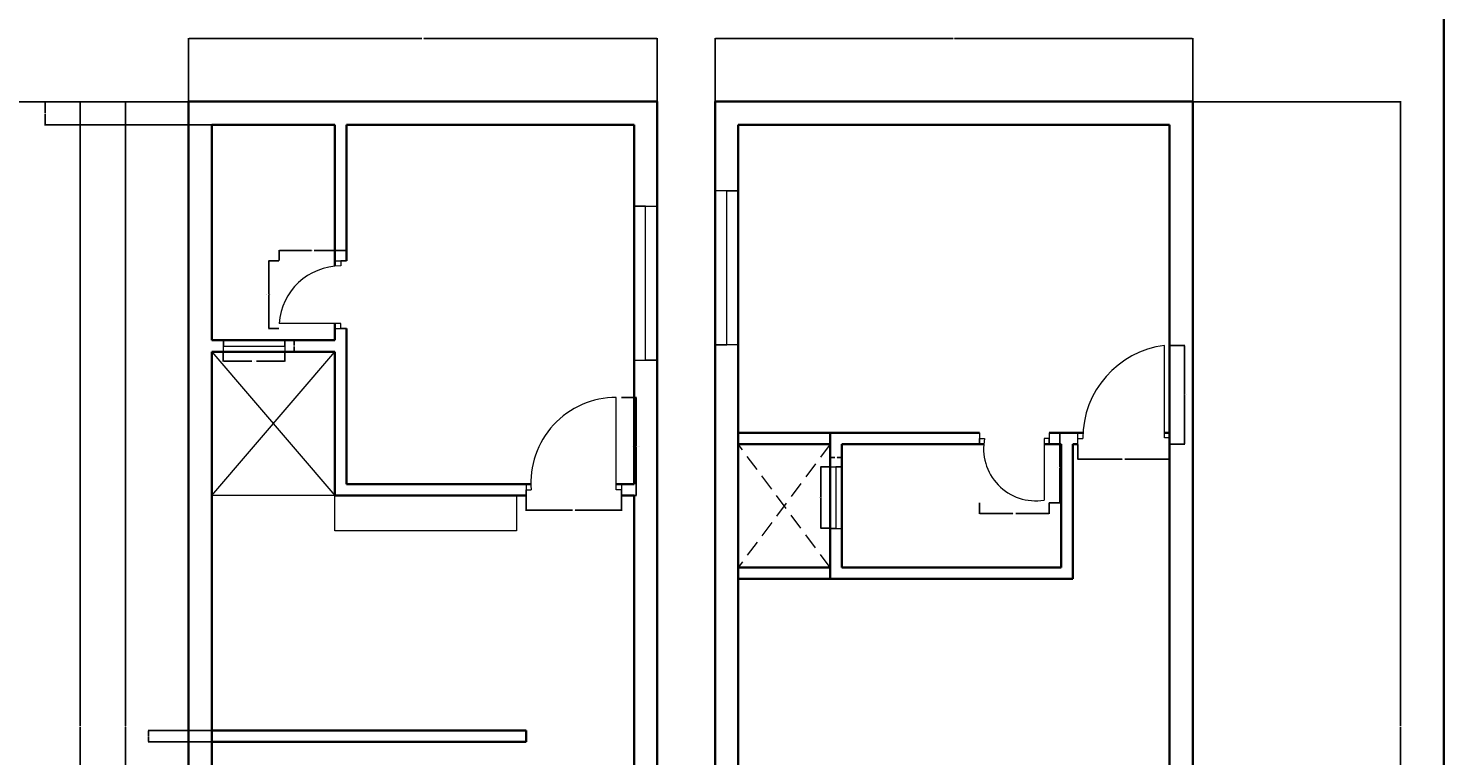
# Model space of a CAD drawing. Units: inches. Extents: x 2169 to 3181, y 1824 to 2912.
# Tile 4 of 5: x 2630 to 3181, y 2163 to 2446. Entities that reach past the tile are written whole.
import ezdxf

# ---------------------------------------------------------------- set-up
doc = ezdxf.new("R2010")
doc.units = ezdxf.units.IN
doc.linetypes.add('DASHED2', pattern=[9.525, 6.35, -3.175])
for name, color, linetype, lineweight in [('A-ANNO-DIMS', 2, 'Continuous', 18), ('A-ANNO-TTLB', 7, 'Continuous', 35), ('A-DOOR', 3, 'Continuous', 18), ('A-FLOR-CASE', 8, 'Continuous', 18), ('A-FLOR-OPEN', 7, 'Continuous', 18), ('A-FLOR-OPEN-OVHD', 253, 'DASHED2', 13), ('A-GLAZ', 4, 'Continuous', 18), ('A-WALL', 7, 'Continuous', 35)]:
    doc.layers.add(name, color=color, linetype=linetype, lineweight=lineweight)
doc.styles.get("Standard").update_dxf_attribs({"font": 'arial.ttf'})
doc.dimstyles.get("Standard").update_dxf_attribs({"dimtxt": 0.18, "dimasz": 0.18, "dimexe": 0.18, "dimexo": 0.0625, "dimgap": 0.09, "dimtad": 0, "dimtih": 1, "dimtoh": 1, "dimdec": 4, "dimzin": 0, "dimdsep": 46, "dimtxsty": 'Standard', "dimcen": 0.09, "dimadec": 0, "dimazin": 0, "dimtfac": 1, "dimtdec": 4, "dimtofl": 0, "dimtmove": 0, "dimatfit": 3, "dimfxl": 1, "dimtolj": 1, "dimtzin": 0, "dimarcsym": 0})

# ---------------------------------------------------------------- blocks, each defined once
blk = doc.blocks.new('DOOR-BED-G-36IN')
for p, q in [((0, 0), (0, 36)), ((-35.15, 2.25), (-35.15, -2.25)), ((2, 2.25), (2, -2.25)), ((-35.15, -2.25), (-35.15, 0)), ((-35.15, 0), (-33.15, 0)), ((2, 0), (0, 0)), ((2, -2.25), (2, 0))]:
    blk.add_line(p, q)
blk.add_arc((0, 2.74), 33.26, 90, 184.7229)
blk = doc.blocks.new('DOOR-BATH-G-24IN')
for p, q in [((-2.25, 24.37), (2.25, 24.37)), ((2.25, 24.37), (0, 24.37)), ((0, 24.37), (0, 22.37)), ((0, 0), (-24, 0)), ((0, -2), (0, 0)), ((-2.25, -2), (-2.25, -2)), ((-2.25, -2), (2.25, -2)), ((2.25, -2), (0, -2))]:
    blk.add_line(p, q)
blk.add_arc((0, -1.69), 24.06, 90, 175.9745)
blk = doc.blocks.new('DOOR-BATH-U-24IN')
for p, q in [((-25.15, 2.25), (-25.15, -2.25)), ((2, 2.25), (2, -2.25)), ((-25.15, -2.25), (-25.15, 0)), ((-25.15, 0), (-23.15, 0)), ((2, 0), (0, 0)), ((0, 0), (0, -24)), ((2, -2.25), (2, 0))]:
    blk.add_line(p, q)
blk.add_arc((-3.27, -3.99), 20.28, 168.6528, 279.2746)
blk = doc.blocks.new('DOOR-BED-U-36IN')
for p, q in [((0, 0), (0, 36)), ((-33.79, -2.49), (-33.79, 2.01)), ((-33.79, 2.01), (-33.79, 2.01)), ((2, 0), (0, 0)), ((-33.79, -0.24), (-31.79, -0.24)), ((-33.79, -2.49), (-33.79, -2.49))]:
    blk.add_line(p, q)
blk.add_arc((4.76, -0.24), 36.56, 97.4851, 180)
blk = doc.blocks.new('WIN-60IN')
for p, q in [((4.5, 60), (0, 60)), ((0, 60), (9, 60)), ((4.5, 0), (4.5, 60)), ((0, 0), (9, 0)), ((9, 0), (4.5, 0)), ((9, 0), (9, 0))]:
    blk.add_line(p, q)
blk = doc.blocks.new('VENT-24IN-G')
for p, q in [((0, 0), (0, 4.5)), ((0, 4.5), (0, 2.25)), ((0, 2.25), (24, 2.25)), ((24, 2.25), (24, 4.5)), ((24, 4.5), (24, 0))]:
    blk.add_line(p, q)
blk = doc.blocks.new('VENT-24IN-U')
for p, q in [((0, 24), (0, 24)), ((0, 24), (4.5, 24)), ((4.5, 24), (2.25, 24)), ((2.25, 24), (2.25, 0)), ((2.25, 0), (0, 0)), ((0, 0), (4.5, 0))]:
    blk.add_line(p, q)
blk = doc.blocks.new('*D23')
at = {"layer": 'A-ANNO-DIMS', "color": 0, "lineweight": -2, "transparency": 16777216}
for p, q in [((2705.49, 2319.83), (2705.49, 2316.11)), ((2705.67, 2316.29), (2716.59, 2316.29)), ((2729.31, 2316.29), (2718.4, 2316.29)), ((2729.49, 2319.83), (2729.49, 2316.11))]:
    blk.add_line(p, q, dxfattribs=at)
at = {"layer": 'A-ANNO-DIMS', "color": 0, "transparency": 16777216}
for points in [[(2705.67, 2316.32), (2705.67, 2316.26), (2705.49, 2316.29)], [(2729.31, 2316.32), (2729.31, 2316.26), (2729.49, 2316.29)]]:
    blk.add_solid(points, dxfattribs=at)
at = {"layer": 'Defpoints', "color": 0, "transparency": 16777216}
for p in [(2705.49, 2319.89), (2729.49, 2319.89), (2729.49, 2316.29)]:
    blk.add_point(p, dxfattribs=at)
at = {"layer": 'A-ANNO-DIMS', "color": 0, "transparency": 16777216, "insert": (2717.49, 2316.29), "char_height": 0.18, "attachment_point": 5}
blk.add_mtext('\\A1;VENT 24 TYP.', dxfattribs=at)
blk = doc.blocks.new('*D24')
at = {"layer": 'A-ANNO-DIMS', "color": 0, "lineweight": -2, "transparency": 16777216}
for p, q in [((2729.56, 2324.39), (2733.27, 2324.39)), ((2733.09, 2324.21), (2733.09, 2322.32)), ((2733.09, 2320.07), (2733.09, 2321.96)), ((2729.56, 2319.89), (2733.27, 2319.89))]:
    blk.add_line(p, q, dxfattribs=at)
at = {"layer": 'A-ANNO-DIMS', "color": 0, "transparency": 16777216}
for points in [[(2733.06, 2324.21), (2733.12, 2324.21), (2733.09, 2324.39)], [(2733.06, 2320.07), (2733.12, 2320.07), (2733.09, 2319.89)]]:
    blk.add_solid(points, dxfattribs=at)
at = {"layer": 'Defpoints', "color": 0, "transparency": 16777216}
for p in [(2729.49, 2324.39), (2733.09, 2324.39), (2729.49, 2319.89)]:
    blk.add_point(p, dxfattribs=at)
at = {"layer": 'A-ANNO-DIMS', "color": 0, "transparency": 16777216, "insert": (2733.09, 2322.14), "char_height": 0.18, "attachment_point": 5}
blk.add_mtext('\\A1;5 TYP.', dxfattribs=at)
blk = doc.blocks.new('*D25')
at = {"layer": 'A-ANNO-DIMS', "color": 0, "lineweight": -2, "transparency": 16777216}
for p, q in [((2941.79, 2275.13), (2938.07, 2275.13)), ((2938.25, 2274.95), (2938.25, 2263.31)), ((2938.25, 2251.31), (2938.25, 2262.95)), ((2941.79, 2251.13), (2938.07, 2251.13))]:
    blk.add_line(p, q, dxfattribs=at)
at = {"layer": 'A-ANNO-DIMS', "color": 0, "transparency": 16777216}
for points in [[(2938.22, 2274.95), (2938.28, 2274.95), (2938.25, 2275.13)], [(2938.22, 2251.31), (2938.28, 2251.31), (2938.25, 2251.13)]]:
    blk.add_solid(points, dxfattribs=at)
at = {"layer": 'Defpoints', "color": 0, "transparency": 16777216}
for p in [(2938.25, 2275.13), (2941.85, 2275.13), (2941.85, 2251.13)]:
    blk.add_point(p, dxfattribs=at)
at = {"layer": 'A-ANNO-DIMS', "color": 0, "transparency": 16777216, "insert": (2938.25, 2263.13), "char_height": 0.18, "attachment_point": 5}
blk.add_mtext('\\A1;VENT 24 TYP.', dxfattribs=at)
blk = doc.blocks.new('*D26')
at = {"layer": 'A-ANNO-DIMS', "color": 0, "lineweight": -2, "transparency": 16777216}
for p, q in [((2941.85, 2275.19), (2941.85, 2278.91)), ((2942.03, 2278.73), (2943.64, 2278.73)), ((2946.17, 2278.73), (2944.56, 2278.73)), ((2946.35, 2275.19), (2946.35, 2278.91))]:
    blk.add_line(p, q, dxfattribs=at)
at = {"layer": 'A-ANNO-DIMS', "color": 0, "transparency": 16777216}
for points in [[(2942.03, 2278.76), (2942.03, 2278.7), (2941.85, 2278.73)], [(2946.17, 2278.76), (2946.17, 2278.7), (2946.35, 2278.73)]]:
    blk.add_solid(points, dxfattribs=at)
at = {"layer": 'Defpoints', "color": 0, "transparency": 16777216}
for p in [(2946.35, 2278.73), (2941.85, 2275.13), (2946.35, 2275.13)]:
    blk.add_point(p, dxfattribs=at)
at = {"layer": 'A-ANNO-DIMS', "color": 0, "transparency": 16777216, "insert": (2944.1, 2278.73), "char_height": 0.18, "attachment_point": 5}
blk.add_mtext('\\A1;5 TYP.', dxfattribs=at)
blk = doc.blocks.new('*D31')
at = {"layer": 'A-ANNO-DIMS', "color": 0, "lineweight": -2, "transparency": 16777216}
for p, q in [((2860.62, 2302.14), (2866.47, 2302.14)), ((2866.29, 2301.96), (2866.29, 2283.2)), ((2866.29, 2264.07), (2866.29, 2282.83)), ((2860.62, 2263.89), (2866.47, 2263.89))]:
    blk.add_line(p, q, dxfattribs=at)
at = {"layer": 'A-ANNO-DIMS', "color": 0, "transparency": 16777216}
for points in [[(2866.26, 2301.96), (2866.32, 2301.96), (2866.29, 2302.14)], [(2866.26, 2264.07), (2866.32, 2264.07), (2866.29, 2263.89)]]:
    blk.add_solid(points, dxfattribs=at)
at = {"layer": 'Defpoints', "color": 0, "transparency": 16777216}
for p in [(2860.56, 2302.14), (2866.29, 2302.14), (2860.56, 2263.89)]:
    blk.add_point(p, dxfattribs=at)
at = {"layer": 'A-ANNO-DIMS', "color": 0, "transparency": 16777216, "insert": (2866.29, 2283.02), "char_height": 0.18, "attachment_point": 5}
blk.add_mtext('\\A1;BEDROOM DOOR 38 TYP.', dxfattribs=at)
blk = doc.blocks.new('*D32')
at = {"layer": 'A-ANNO-DIMS', "color": 0, "lineweight": -2, "transparency": 16777216}
for p, q in [((2823.41, 2263.83), (2823.41, 2257.97)), ((2860.56, 2263.83), (2860.56, 2257.97)), ((2823.59, 2258.15), (2841.45, 2258.15)), ((2860.38, 2258.15), (2842.51, 2258.15))]:
    blk.add_line(p, q, dxfattribs=at)
at = {"layer": 'A-ANNO-DIMS', "color": 0, "transparency": 16777216}
for points in [[(2823.59, 2258.18), (2823.59, 2258.12), (2823.41, 2258.15)], [(2860.38, 2258.18), (2860.38, 2258.12), (2860.56, 2258.15)]]:
    blk.add_solid(points, dxfattribs=at)
at = {"layer": 'Defpoints', "color": 0, "transparency": 16777216}
for p in [(2823.41, 2263.89), (2860.56, 2263.89), (2860.56, 2258.15)]:
    blk.add_point(p, dxfattribs=at)
at = {"layer": 'A-ANNO-DIMS', "color": 0, "transparency": 16777216, "insert": (2841.98, 2258.15), "char_height": 0.18, "attachment_point": 5}
blk.add_mtext('\\A1;37 TYP.', dxfattribs=at)
blk = doc.blocks.new('*D33')
at = {"layer": 'A-ANNO-DIMS', "color": 0, "lineweight": -2, "transparency": 16777216}
for p, q in [((2727.14, 2355.37), (2723.07, 2355.37)), ((2723.25, 2355.19), (2723.25, 2342.37)), ((2723.25, 2329.18), (2723.25, 2342)), ((2727.14, 2329), (2723.07, 2329))]:
    blk.add_line(p, q, dxfattribs=at)
at = {"layer": 'A-ANNO-DIMS', "color": 0, "transparency": 16777216}
for points in [[(2723.22, 2355.19), (2723.28, 2355.19), (2723.25, 2355.37)], [(2723.22, 2329.18), (2723.28, 2329.18), (2723.25, 2329)]]:
    blk.add_solid(points, dxfattribs=at)
at = {"layer": 'Defpoints', "color": 0, "transparency": 16777216}
for p in [(2723.25, 2355.37), (2727.21, 2355.37), (2727.21, 2329)]:
    blk.add_point(p, dxfattribs=at)
at = {"layer": 'A-ANNO-DIMS', "color": 0, "transparency": 16777216, "insert": (2723.25, 2342.19), "char_height": 0.18, "attachment_point": 5}
blk.add_mtext('\\A1;WC DOOR 26 TYP.', dxfattribs=at)
blk = doc.blocks.new('*D34')
at = {"layer": 'A-ANNO-DIMS', "color": 0, "lineweight": -2, "transparency": 16777216}
for p, q in [((2727.21, 2355.44), (2727.21, 2359.51)), ((2727.39, 2359.33), (2739.8, 2359.33)), ((2753.28, 2359.33), (2740.86, 2359.33)), ((2753.46, 2355.44), (2753.46, 2359.51))]:
    blk.add_line(p, q, dxfattribs=at)
at = {"layer": 'A-ANNO-DIMS', "color": 0, "transparency": 16777216}
for points in [[(2727.39, 2359.36), (2727.39, 2359.3), (2727.21, 2359.33)], [(2753.28, 2359.36), (2753.28, 2359.3), (2753.46, 2359.33)]]:
    blk.add_solid(points, dxfattribs=at)
at = {"layer": 'Defpoints', "color": 0, "transparency": 16777216}
for p in [(2727.21, 2355.37), (2753.46, 2359.33), (2753.46, 2355.37)]:
    blk.add_point(p, dxfattribs=at)
at = {"layer": 'A-ANNO-DIMS', "color": 0, "transparency": 16777216, "insert": (2740.33, 2359.33), "char_height": 0.18, "attachment_point": 5}
blk.add_mtext('\\A1;26 TYP.', dxfattribs=at)
blk = doc.blocks.new('*D37')
at = {"layer": 'A-ANNO-DIMS', "color": 0, "lineweight": -2, "transparency": 16777216}
for p, q in [((3074.12, 2322.39), (3080.01, 2322.39)), ((3079.83, 2322.21), (3079.83, 2303.32)), ((3079.83, 2284.07), (3079.83, 2302.96)), ((3074.12, 2283.89), (3080.01, 2283.89))]:
    blk.add_line(p, q, dxfattribs=at)
at = {"layer": 'A-ANNO-DIMS', "color": 0, "transparency": 16777216}
for points in [[(3079.8, 2322.21), (3079.86, 2322.21), (3079.83, 2322.39)], [(3079.8, 2284.07), (3079.86, 2284.07), (3079.83, 2283.89)]]:
    blk.add_solid(points, dxfattribs=at)
at = {"layer": 'Defpoints', "color": 0, "transparency": 16777216}
for p in [(3074.05, 2322.39), (3079.83, 2322.39), (3074.05, 2283.89)]:
    blk.add_point(p, dxfattribs=at)
at = {"layer": 'A-ANNO-DIMS', "color": 0, "transparency": 16777216, "insert": (3079.83, 2303.14), "char_height": 0.18, "attachment_point": 5}
blk.add_mtext('\\A1;BEDROOM DOOR 38 TYP.', dxfattribs=at)
blk = doc.blocks.new('*D38')
at = {"layer": 'A-ANNO-DIMS', "color": 0, "lineweight": -2, "transparency": 16777216}
for p, q in [((3038.26, 2283.83), (3038.26, 2277.94)), ((3074.05, 2283.83), (3074.05, 2277.94)), ((3038.44, 2278.12), (3055.63, 2278.12)), ((3073.87, 2278.12), (3056.68, 2278.12))]:
    blk.add_line(p, q, dxfattribs=at)
at = {"layer": 'A-ANNO-DIMS', "color": 0, "transparency": 16777216}
for points in [[(3038.44, 2278.15), (3038.44, 2278.09), (3038.26, 2278.12)], [(3073.87, 2278.15), (3073.87, 2278.09), (3074.05, 2278.12)]]:
    blk.add_solid(points, dxfattribs=at)
at = {"layer": 'Defpoints', "color": 0, "transparency": 16777216}
for p in [(3038.26, 2283.89), (3074.05, 2283.89), (3074.05, 2278.12)]:
    blk.add_point(p, dxfattribs=at)
at = {"layer": 'A-ANNO-DIMS', "color": 0, "transparency": 16777216, "insert": (3056.16, 2278.12), "char_height": 0.18, "attachment_point": 5}
blk.add_mtext('\\A1;36 TYP.', dxfattribs=at)
blk = doc.blocks.new('*D39')
at = {"layer": 'A-ANNO-DIMS', "color": 0, "lineweight": -2, "transparency": 16777216}
for p, q in [((3027.22, 2288.39), (3031.44, 2288.39)), ((3031.26, 2288.21), (3031.26, 2274.91)), ((3031.26, 2261.25), (3031.26, 2274.55)), ((3027.22, 2261.07), (3031.44, 2261.07))]:
    blk.add_line(p, q, dxfattribs=at)
at = {"layer": 'A-ANNO-DIMS', "color": 0, "transparency": 16777216}
for points in [[(3031.23, 2288.21), (3031.29, 2288.21), (3031.26, 2288.39)], [(3031.23, 2261.25), (3031.29, 2261.25), (3031.26, 2261.07)]]:
    blk.add_solid(points, dxfattribs=at)
at = {"layer": 'Defpoints', "color": 0, "transparency": 16777216}
for p in [(3027.16, 2288.39), (3031.26, 2288.39), (3027.16, 2261.07)]:
    blk.add_point(p, dxfattribs=at)
at = {"layer": 'A-ANNO-DIMS', "color": 0, "transparency": 16777216, "insert": (3031.26, 2274.73), "char_height": 0.18, "attachment_point": 5}
blk.add_mtext('\\A1;WC DOOR 27 TYP.', dxfattribs=at)
blk = doc.blocks.new('*D40')
at = {"layer": 'A-ANNO-DIMS', "color": 0, "lineweight": -2, "transparency": 16777216}
for p, q in [((3000.01, 2261.01), (3000.01, 2256.79)), ((3027.16, 2261.01), (3027.16, 2256.79)), ((3000.19, 2256.97), (3013.06, 2256.97)), ((3026.98, 2256.97), (3014.12, 2256.97))]:
    blk.add_line(p, q, dxfattribs=at)
at = {"layer": 'A-ANNO-DIMS', "color": 0, "transparency": 16777216}
for points in [[(3000.19, 2257), (3000.19, 2256.94), (3000.01, 2256.97)], [(3026.98, 2257), (3026.98, 2256.94), (3027.16, 2256.97)]]:
    blk.add_solid(points, dxfattribs=at)
at = {"layer": 'Defpoints', "color": 0, "transparency": 16777216}
for p in [(3000.01, 2261.07), (3027.16, 2261.07), (3027.16, 2256.97)]:
    blk.add_point(p, dxfattribs=at)
at = {"layer": 'A-ANNO-DIMS', "color": 0, "transparency": 16777216, "insert": (3013.59, 2256.97), "char_height": 0.18, "attachment_point": 5}
blk.add_mtext('\\A1;27 TYP.', dxfattribs=at)
blk = doc.blocks.new('*D56')
at = {"layer": 'A-ANNO-DIMS', "color": 0, "lineweight": -2, "transparency": 16777216}
for p, q in [((2623.43, 2417.39), (2649.9, 2417.39)), ((2649.72, 2417.21), (2649.72, 2174.07)), ((2649.72, 1930.57), (2649.72, 2173.71)), ((2623.43, 1930.39), (2649.9, 1930.39))]:
    blk.add_line(p, q, dxfattribs=at)
at = {"layer": 'A-ANNO-DIMS', "color": 0, "transparency": 16777216}
for points in [[(2649.69, 2417.21), (2649.75, 2417.21), (2649.72, 2417.39)], [(2649.69, 1930.57), (2649.75, 1930.57), (2649.72, 1930.39)]]:
    blk.add_solid(points, dxfattribs=at)
at = {"layer": 'Defpoints', "color": 0, "transparency": 16777216}
for p in [(2623.37, 2417.39), (2649.72, 2417.39), (2623.37, 1930.39)]:
    blk.add_point(p, dxfattribs=at)
at = {"layer": 'A-ANNO-DIMS', "color": 0, "transparency": 16777216, "insert": (2649.72, 2173.89), "char_height": 0.18, "attachment_point": 5}
blk.add_mtext('\\A1;487', dxfattribs=at)
blk = doc.blocks.new('*D64')
at = {"layer": 'A-ANNO-DIMS', "color": 0, "lineweight": -2, "transparency": 16777216}
for p, q in [((2691.96, 2417.45), (2691.96, 2442.17)), ((2692.14, 2441.99), (2782.82, 2441.99)), ((2874.28, 2441.99), (2783.59, 2441.99)), ((2874.46, 2417.45), (2874.46, 2442.17))]:
    blk.add_line(p, q, dxfattribs=at)
at = {"layer": 'A-ANNO-DIMS', "color": 0, "transparency": 16777216}
for points in [[(2692.14, 2442.02), (2692.14, 2441.96), (2691.96, 2441.99)], [(2874.28, 2442.02), (2874.28, 2441.96), (2874.46, 2441.99)]]:
    blk.add_solid(points, dxfattribs=at)
at = {"layer": 'Defpoints', "color": 0, "transparency": 16777216}
for p in [(2874.46, 2441.99), (2691.96, 2417.39), (2874.46, 2417.39)]:
    blk.add_point(p, dxfattribs=at)
at = {"layer": 'A-ANNO-DIMS', "color": 0, "transparency": 16777216, "insert": (2783.21, 2441.99), "char_height": 0.18, "attachment_point": 5}
blk.add_mtext('\\A1;182.5', dxfattribs=at)
blk = doc.blocks.new('*D65')
at = {"layer": 'A-ANNO-DIMS', "color": 0, "lineweight": -2, "transparency": 16777216}
for p, q in [((2691.89, 2417.39), (2667.18, 2417.39)), ((2667.36, 2417.21), (2667.36, 2174.07)), ((2667.36, 1930.57), (2667.36, 2173.71)), ((2691.89, 1930.39), (2667.18, 1930.39))]:
    blk.add_line(p, q, dxfattribs=at)
at = {"layer": 'A-ANNO-DIMS', "color": 0, "transparency": 16777216}
for points in [[(2667.33, 2417.21), (2667.39, 2417.21), (2667.36, 2417.39)], [(2667.33, 1930.57), (2667.39, 1930.57), (2667.36, 1930.39)]]:
    blk.add_solid(points, dxfattribs=at)
at = {"layer": 'Defpoints', "color": 0, "transparency": 16777216}
for p in [(2667.36, 2417.39), (2691.96, 2417.39), (2691.96, 1930.39)]:
    blk.add_point(p, dxfattribs=at)
at = {"layer": 'A-ANNO-DIMS', "color": 0, "transparency": 16777216, "insert": (2667.36, 2173.89), "char_height": 0.18, "attachment_point": 5}
blk.add_mtext('\\A1;487', dxfattribs=at)
blk = doc.blocks.new('*D66')
at = {"layer": 'A-ANNO-DIMS', "color": 0, "lineweight": -2, "transparency": 16777216}
for p, q in [((2897.05, 2417.45), (2897.05, 2442.17)), ((2897.23, 2441.99), (2989.77, 2441.99)), ((3082.87, 2441.99), (2990.33, 2441.99)), ((3083.05, 2417.45), (3083.05, 2442.17))]:
    blk.add_line(p, q, dxfattribs=at)
at = {"layer": 'A-ANNO-DIMS', "color": 0, "transparency": 16777216}
for points in [[(2897.23, 2442.02), (2897.23, 2441.96), (2897.05, 2441.99)], [(3082.87, 2442.02), (3082.87, 2441.96), (3083.05, 2441.99)]]:
    blk.add_solid(points, dxfattribs=at)
at = {"layer": 'Defpoints', "color": 0, "transparency": 16777216}
for p in [(3083.05, 2441.99), (2897.05, 2417.39), (3083.05, 2417.39)]:
    blk.add_point(p, dxfattribs=at)
at = {"layer": 'A-ANNO-DIMS', "color": 0, "transparency": 16777216, "insert": (2990.05, 2441.99), "char_height": 0.18, "attachment_point": 5}
blk.add_mtext('\\A1;186', dxfattribs=at)
blk = doc.blocks.new('*D67')
at = {"layer": 'A-ANNO-DIMS', "color": 0, "lineweight": -2, "transparency": 16777216}
for p, q in [((3083.12, 2417.39), (3164.24, 2417.39)), ((3164.06, 2417.21), (3164.06, 2174.07)), ((3164.06, 1930.57), (3164.06, 2173.71)), ((3083.12, 1930.39), (3164.24, 1930.39))]:
    blk.add_line(p, q, dxfattribs=at)
at = {"layer": 'A-ANNO-DIMS', "color": 0, "transparency": 16777216}
for points in [[(3164.03, 2417.21), (3164.09, 2417.21), (3164.06, 2417.39)], [(3164.03, 1930.57), (3164.09, 1930.57), (3164.06, 1930.39)]]:
    blk.add_solid(points, dxfattribs=at)
at = {"layer": 'Defpoints', "color": 0, "transparency": 16777216}
for p in [(3083.05, 2417.39), (3164.06, 2417.39), (3083.05, 1930.39)]:
    blk.add_point(p, dxfattribs=at)
at = {"layer": 'A-ANNO-DIMS', "color": 0, "transparency": 16777216, "insert": (3164.06, 2173.89), "char_height": 0.18, "attachment_point": 5}
blk.add_mtext('\\A1;487', dxfattribs=at)
blk = doc.blocks.new('*D69')
at = {"layer": 'A-ANNO-DIMS', "color": 0, "lineweight": -2, "transparency": 16777216}
for p, q in [((2691.89, 2417.39), (2635.88, 2417.39)), ((2636.06, 2417.21), (2636.06, 2413.07)), ((2636.06, 2408.57), (2636.06, 2412.71)), ((2700.89, 2408.39), (2635.88, 2408.39))]:
    blk.add_line(p, q, dxfattribs=at)
at = {"layer": 'A-ANNO-DIMS', "color": 0, "transparency": 16777216}
for points in [[(2636.03, 2417.21), (2636.09, 2417.21), (2636.06, 2417.39)], [(2636.03, 2408.57), (2636.09, 2408.57), (2636.06, 2408.39)]]:
    blk.add_solid(points, dxfattribs=at)
at = {"layer": 'Defpoints', "color": 0, "transparency": 16777216}
for p in [(2691.96, 2417.39), (2636.06, 2408.39), (2700.96, 2408.39)]:
    blk.add_point(p, dxfattribs=at)
at = {"layer": 'A-ANNO-DIMS', "color": 0, "transparency": 16777216, "insert": (2636.06, 2412.89), "char_height": 0.18, "attachment_point": 5}
blk.add_mtext('\\A1;9', dxfattribs=at)
blk = doc.blocks.new('*D70')
at = {"layer": 'A-ANNO-DIMS', "color": 0, "lineweight": -2, "transparency": 16777216}
for p, q in [((2700.89, 2172.39), (2676.18, 2172.39)), ((2676.36, 2172.21), (2676.36, 2170.32)), ((2700.89, 2167.89), (2676.18, 2167.89)), ((2676.36, 2168.07), (2676.36, 2169.96))]:
    blk.add_line(p, q, dxfattribs=at)
at = {"layer": 'A-ANNO-DIMS', "color": 0, "transparency": 16777216}
for points in [[(2676.33, 2172.21), (2676.39, 2172.21), (2676.36, 2172.39)], [(2676.33, 2168.07), (2676.39, 2168.07), (2676.36, 2167.89)]]:
    blk.add_solid(points, dxfattribs=at)
at = {"layer": 'Defpoints', "color": 0, "transparency": 16777216}
for p in [(2676.36, 2172.39), (2700.96, 2172.39), (2700.96, 2167.89)]:
    blk.add_point(p, dxfattribs=at)
at = {"layer": 'A-ANNO-DIMS', "color": 0, "transparency": 16777216, "insert": (2676.36, 2170.14), "char_height": 0.18, "attachment_point": 5}
blk.add_mtext('\\A1;4.5', dxfattribs=at)

msp = doc.modelspace()

# ---------------------------------------------------------------- linework, layer by layer
at = {"layer": 'A-ANNO-TTLB'}
msp.add_lwpolyline([(2168.7598, 2912.462), (3180.8253, 2912.462), (3180.8253, 1823.5481), (2168.7598, 1823.5481)], close=True, dxfattribs=at)
at = {"layer": 'A-FLOR-CASE'}
msp.add_lwpolyline([(2748.9572, 2263.8924), (2819.6652, 2263.8924), (2819.6652, 2250.1381), (2748.9572, 2250.1381)], close=True, dxfattribs=at)
at = {"layer": 'A-FLOR-OPEN'}
for p, q in [((2700.9572, 2263.8924), (2748.9572, 2319.8924)), ((2700.9572, 2319.8924), (2748.9572, 2263.8924)), ((2748.9572, 2263.8924), (2700.9572, 2263.8924))]:
    msp.add_line(p, q, dxfattribs=at)
at = {"layer": 'A-FLOR-OPEN-OVHD'}
for p, q in [((2941.8523, 2283.8924), (2906.0534, 2235.8924)), ((2941.8523, 2235.8924), (2906.0534, 2283.8924)), ((2941.8523, 2273.085), (2941.8523, 2273.085))]:
    msp.add_line(p, q, dxfattribs=at)
at = {"layer": 'A-WALL'}
for p, q in [((2691.9572, 2417.3924), (2874.4572, 2417.3924)), ((2691.9572, 2417.3924), (2874.4572, 2417.3924)), ((2691.9572, 2417.3924), (2691.9572, 1930.3924)), ((2874.4572, 2417.3924), (2874.4572, 1930.3924)), ((2897.0534, 2417.3924), (3083.0534, 2417.3924)), ((2897.0534, 2417.3924), (2897.0534, 1930.3924)), ((3074.0534, 2417.3924), (3083.0534, 2417.3924)), ((3083.0534, 2417.3924), (3083.0534, 1930.3924)), ((2700.9572, 2408.3924), (2748.9572, 2408.3924)), ((2700.9572, 2408.3924), (2700.9572, 2324.3924)), ((2748.9572, 2408.3924), (2748.9572, 2353.2673)), ((2753.4572, 2408.3924), (2865.4572, 2408.3924)), ((2753.4572, 2408.3924), (2753.4572, 2355.3727)), ((2865.4572, 2408.3924), (2865.4572, 2268.3924)), ((2906.0534, 2408.3924), (3074.0534, 2408.3924)), ((2906.0534, 2408.3924), (2906.0534, 2023.8924)), ((2906.0534, 2408.3924), (3070.0534, 2408.3924)), ((2906.0534, 2408.3924), (3074.0534, 2408.3924)), ((3074.0534, 2408.3924), (3074.0534, 1930.3924)), ((2748.9572, 2331.0023), (2748.9572, 2324.3924)), ((2753.4572, 2329.0023), (2753.4572, 2268.3924)), ((2700.9572, 2324.3924), (2748.9572, 2324.3924)), ((2700.9572, 2319.8924), (2748.9572, 2319.8924)), ((2700.9572, 2319.8924), (2700.9572, 2023.8924)), ((2748.9572, 2319.8924), (2748.9572, 2263.8924)), ((2941.8523, 2288.3924), (2906.0534, 2288.3924)), ((2906.0534, 2288.3924), (2906.0534, 2283.8924)), ((2941.8523, 2288.3924), (3000.0137, 2288.3924)), ((2941.8523, 2288.3924), (2941.8523, 2231.3924)), ((2941.8523, 2288.3924), (3000.0137, 2288.3924)), ((3027.1608, 2288.3924), (3040.3285, 2288.3924)), ((3027.1608, 2288.3924), (3031.8523, 2288.3924)), ((3072.0534, 2288.3924), (3074.0534, 2288.3924)), ((2906.0534, 2283.8924), (2941.8523, 2283.8924)), ((2906.0534, 2283.8924), (2910.5534, 2283.8924)), ((2941.8523, 2283.8924), (2941.8523, 2231.3924)), ((2946.3523, 2283.8924), (3001.6921, 2283.8924)), ((2946.3523, 2283.8924), (2946.3523, 2235.8924)), ((3025.1608, 2283.8924), (3031.8523, 2283.8924)), ((3031.8523, 2283.8924), (3031.8523, 2235.8924)), ((3036.3523, 2283.8924), (3038.2592, 2283.8924)), ((3036.3523, 2231.3924), (3036.3523, 2283.8924)), ((2753.4572, 2268.3924), (2825.2991, 2268.3924)), ((2858.5569, 2268.3924), (2865.4572, 2268.3924)), ((2748.9572, 2263.8924), (2823.4085, 2263.8924)), ((2860.5569, 2263.8924), (2865.4572, 2263.8924)), ((2865.4572, 2263.8924), (2865.4572, 1930.3924)), ((2906.0534, 2231.3924), (2906.0534, 2235.8924)), ((2906.0534, 2235.8924), (2941.8523, 2235.8924)), ((2941.8523, 2235.8924), (2941.8523, 2235.8924)), ((2946.3523, 2235.8924), (3031.8523, 2235.8924)), ((2941.8523, 2231.3924), (2906.0534, 2231.3924)), ((2941.8523, 2231.3924), (3036.3523, 2231.3924)), ((3031.8523, 2231.3924), (3036.3523, 2231.3924)), ((2700.9572, 2172.3924), (2823.4085, 2172.3924)), ((2823.4085, 2172.3924), (2823.4085, 2167.8924)), ((2700.9572, 2167.8924), (2823.4085, 2167.8924))]:
    msp.add_line(p, q, dxfattribs=at)

# ---------------------------------------------------------------- block references
at = {"layer": 'A-DOOR'}
for name, p in [('DOOR-BATH-G-24IN', (2751.2072, 2331.0023)), ('DOOR-BED-U-36IN', (3072.0534, 2286.3872)), ('DOOR-BED-G-36IN', (2858.5569, 2266.1424)), ('DOOR-BATH-U-24IN', (3025.1608, 2286.1424))]:
    msp.add_blockref(name, p, dxfattribs=at)
at = {"layer": 'A-GLAZ', "extrusion": (0, 0, -1), "zscale": -1}
msp.add_blockref('WIN-60IN', (-2906.053, 2322.6361), dxfattribs=at)
at = {"layer": 'A-GLAZ'}
for name, p in [('WIN-60IN', (2865.4576, 2316.692)), ('VENT-24IN-G', (2705.4926, 2319.892)), ('VENT-24IN-U', (2941.8526, 2251.127))]:
    msp.add_blockref(name, p, dxfattribs=at)

# ---------------------------------------------------------------- dimensions: what is measured, and where the dimension line sits
at = {"layer": 'A-ANNO-DIMS'}
for base, p1, p2, override, picture, middle in [((2874.4572, 2441.9924), (2691.9572, 2417.3924), (2874.4572, 2417.3924), {"dimdec": 1, "dimlfac": 1, "dimrnd": 0, "dimzin": 0, "dimdsep": 46, "dimlunit": 2}, '*D64', (2783.2072, 2441.9924)), ((3083.0534, 2441.9924), (2897.0534, 2417.3924), (3083.0534, 2417.3924), {"dimdec": 0, "dimlfac": 1, "dimrnd": 0, "dimzin": 0, "dimdsep": 46, "dimlunit": 2}, '*D66', (2990.0534, 2441.9924))]:
    dim = msp.add_linear_dim(base=base, p1=p1, p2=p2, dimstyle='Standard', override=override, dxfattribs=at)
    dim.commit()
    dim.dimension.update_dxf_attribs({"geometry": picture, "text_midpoint": middle})
for base, p1, p2, override, picture, middle in [((2649.7198, 2417.3924), (2623.3698, 1930.3924), (2623.3698, 2417.3924), {"dimdec": 0, "dimlfac": 1, "dimrnd": 0, "dimzin": 0, "dimdsep": 46, "dimlunit": 2}, '*D56', (2649.7198, 2173.8924)), ((2636.0608, 2408.3924), (2691.9572, 2417.3924), (2700.9572, 2408.3924), {"dimdec": 0, "dimlfac": 1, "dimrnd": 0, "dimzin": 0, "dimdsep": 46, "dimlunit": 2}, '*D69', (2636.0608, 2412.8924)), ((2667.3572, 2417.3924), (2691.9572, 1930.3924), (2691.9572, 2417.3924), {"dimdec": 0, "dimlfac": 1, "dimrnd": 0, "dimzin": 0, "dimdsep": 46, "dimlunit": 2}, '*D65', (2667.3572, 2173.8924)), ((3164.0639, 2417.3924), (3083.0534, 1930.3924), (3083.0534, 2417.3924), {"dimdec": 0, "dimlfac": 1, "dimrnd": 0, "dimzin": 0, "dimdsep": 46, "dimlunit": 2}, '*D67', (3164.0639, 2173.8924)), ((2676.3572, 2172.3924), (2700.9572, 2167.8924), (2700.9572, 2172.3924), {"dimdec": 1, "dimlfac": 1, "dimrnd": 0, "dimzin": 0, "dimdsep": 46, "dimlunit": 2}, '*D70', (2676.3572, 2170.1424))]:
    dim = msp.add_linear_dim(base=base, p1=p1, p2=p2, angle=90, dimstyle='Standard', override=override, dxfattribs=at)
    dim.commit()
    dim.dimension.update_dxf_attribs({"geometry": picture, "text_midpoint": middle})
for base, p1, p2, text, picture, middle in [((2753.4572, 2359.3283), (2727.2072, 2355.3727), (2753.4572, 2355.3727), '<> TYP.', '*D34', (2740.3322, 2359.3283)), ((2729.4928, 2316.2924), (2705.4928, 2319.8924), (2729.4928, 2319.8924), 'VENT <> TYP.', '*D23', (2717.4928, 2316.2924)), ((3074.0534, 2278.1182), (3038.2592, 2283.8924), (3074.0534, 2283.8924), '<> TYP.', '*D38', (3056.1563, 2278.1182)), ((2946.3522891072, 2278.7265913297), (2941.8522891072, 2275.1265913297), (2946.3522891072, 2275.1265913297), '<> TYP.', '*D26', (2944.1022891072, 2278.7265913297)), ((2860.5569, 2258.1549), (2823.4085, 2263.8924), (2860.5569, 2263.8924), '<> TYP.', '*D32', (2841.9827, 2258.1549)), ((3027.1608, 2256.9716), (3000.0137, 2261.07), (3027.1608, 2261.07), '<> TYP.', '*D40', (3013.5873, 2256.9716))]:
    dim = msp.add_linear_dim(base=base, p1=p1, p2=p2, text=text, dimstyle='Standard', override={"dimdec": 0, "dimlfac": 1, "dimrnd": 0, "dimzin": 0, "dimdsep": 46, "dimlunit": 2}, dxfattribs=at)
    dim.commit()
    dim.dimension.update_dxf_attribs({"geometry": picture, "text_midpoint": middle})
for base, p1, p2, text, picture, middle in [((2723.2517, 2355.3727), (2727.2072, 2329.0023), (2727.2072, 2355.3727), 'WC DOOR <> TYP.', '*D33', (2723.2517, 2342.1875)), ((2733.0927991291, 2324.3923951293), (2729.4927991291, 2319.8923951293), (2729.4927991291, 2324.3923951293), '<> TYP.', '*D24', (2733.0927991291, 2322.1423951293)), ((3079.8276, 2322.3872), (3074.0534, 2283.8924), (3074.0534, 2322.3872), 'BEDROOM DOOR <> TYP.', '*D37', (3079.8276, 2303.1398)), ((2866.2944, 2302.1424), (2860.5569, 2263.8924), (2860.5569, 2302.1424), 'BEDROOM DOOR <> TYP.', '*D31', (2866.2944, 2283.0174)), ((3031.2592, 2288.3924), (3027.1608, 2261.07), (3027.1608, 2288.3924), 'WC DOOR <> TYP.', '*D39', (3031.2592, 2274.7312)), ((2938.2523, 2275.1266), (2941.8523, 2251.1266), (2941.8523, 2275.1266), 'VENT <> TYP.', '*D25', (2938.2523, 2263.1266))]:
    dim = msp.add_linear_dim(base=base, p1=p1, p2=p2, angle=90, text=text, dimstyle='Standard', override={"dimdec": 0, "dimlfac": 1, "dimrnd": 0, "dimzin": 0, "dimdsep": 46, "dimlunit": 2}, dxfattribs=at)
    dim.commit()
    dim.dimension.update_dxf_attribs({"geometry": picture, "text_midpoint": middle})

doc.saveas('drawing.dxf')
